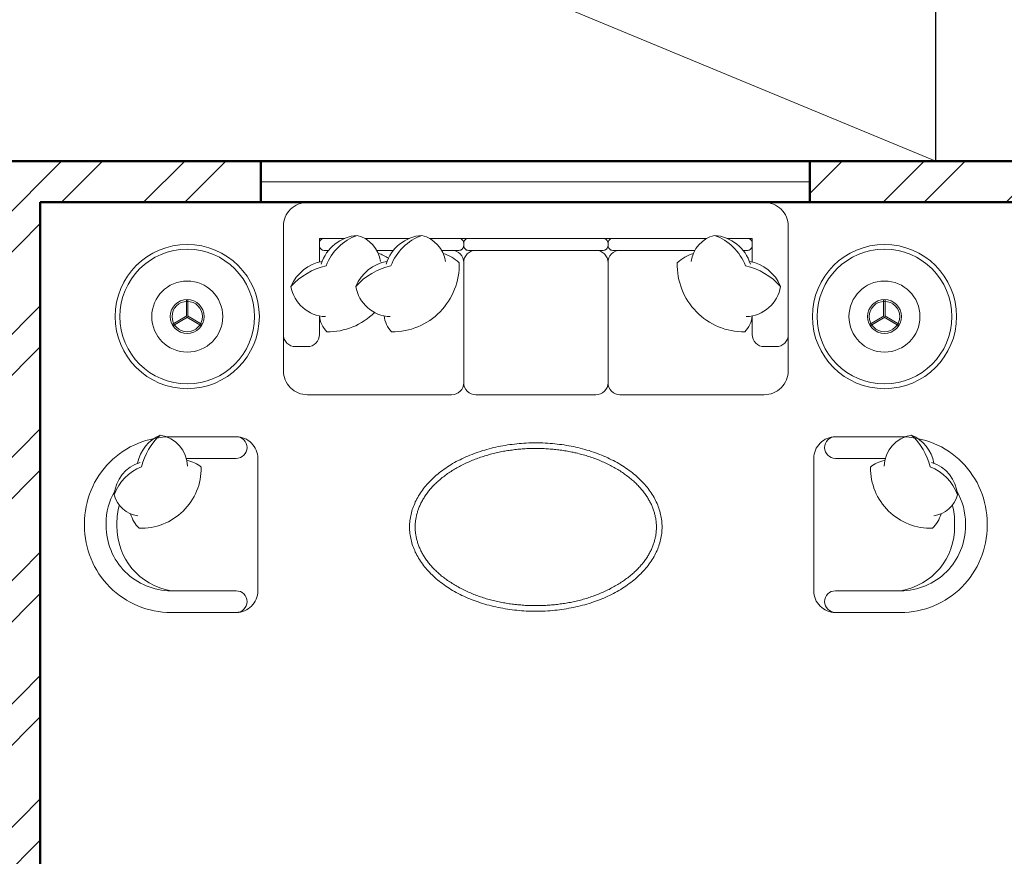
# Model space of a CAD drawing. Units: inches. Extents: x 1901 to 2863, y 888 to 2433.
# Tile 19 of 91: x 2157 to 2264, y 1641 to 1732. Entities that reach past the tile are written whole.
import ezdxf

# ---------------------------------------------------------------- set-up
doc = ezdxf.new("R2010")
doc.units = ezdxf.units.IN
for name, color, linetype, lineweight in [('A-ANNO-SYMB', 8, 'Continuous', 13), ('A-FLOR-HRAL', 41, 'Continuous', 25), ('A-FURN', 8, 'Continuous', 18), ('A-WALL', 7, 'Continuous', 50), ('A-WALL-PATT', 8, 'Continuous', 13)]:
    doc.layers.add(name, color=color, linetype=linetype, lineweight=lineweight)

msp = doc.modelspace()

# ---------------------------------------------------------------- hatches: boundary and pattern name
at = {"layer": 'A-WALL-PATT'}
h = msp.add_hatch(dxfattribs=at)
h.set_pattern_fill('ANSI32', color=256)
h.paths.add_polyline_path([(2182.93, 1716.63), (2024.93, 1716.63), (2024.93, 1681.7), (2029.33, 1681.7), (2029.33, 1712.13), (2154.33, 1712.13), (2154.33, 1580.13), (2148.52, 1580.13), (2148.52, 1577.88), (2148.52, 1575.63), (2194.93, 1575.63), (2194.93, 1580.13), (2158.83, 1580.13), (2158.83, 1712.13), (2182.93, 1712.13)])
h.paths.add_polyline_path([(2301.07, 1716.63), (2242.93, 1716.63), (2242.93, 1712.13), (2283.83, 1712.13), (2283.83, 1685.54), (2288.33, 1685.54), (2288.33, 1712.13), (2301.07, 1712.13)])
h.paths.add_polyline_path([(2288.33, 1600.41), (2286.08, 1600.41), (2283.83, 1600.41), (2283.83, 1580.13), (2270.6, 1580.13), (2270.6, 1575.63), (2288.33, 1575.63)])
h.paths.add_polyline_path([(2295.93, 1953.63), (2271.45, 1953.63), (2271.45, 1949.13), (2291.43, 1949.13), (2291.43, 1941.24), (2295.93, 1941.24)])
h.paths.add_polyline_path([(2098.38, 1244.13), (2082.33, 1244.13), (2082.33, 1302.13), (2086.52, 1302.13), (2086.52, 1306.63), (2067.46, 1306.63), (2067.46, 1302.13), (2077.83, 1302.13), (2077.83, 1239.63), (2098.38, 1239.63), (2098.38, 1241.88)])
h.paths.add_polyline_path([(2217.31, 1306.63), (2158.83, 1306.63), (2158.83, 1451.63), (2162.72, 1451.63), (2162.72, 1453.88), (2162.72, 1456.13), (2154.33, 1456.13), (2154.33, 1443.13), (2151.91, 1443.13), (2151.91, 1438.63), (2154.33, 1438.63), (2154.33, 1306.63), (2109.31, 1306.63), (2109.31, 1304.38), (2109.31, 1302.13), (2154.33, 1302.13), (2154.33, 1244.13), (2122.38, 1244.13), (2122.38, 1239.63), (2154.33, 1239.63), (2154.33, 1223.63), (2163.33, 1223.63), (2181.01, 1223.63), (2181.01, 1225.88), (2181.01, 1228.13), (2163.33, 1228.13), (2163.33, 1258.22), (2158.83, 1258.22), (2158.83, 1302.13), (2217.31, 1302.13)])
h.paths.add_polyline_path([(2259.99, 1306.63), (2238.3, 1306.63), (2238.3, 1304.38), (2238.3, 1302.13), (2242.83, 1302.13), (2242.83, 1228.13), (2205.01, 1228.13), (2205.01, 1223.63), (2247.33, 1223.63), (2247.33, 1302.13), (2259.99, 1302.13), (2259.99, 1304.38)])
h.paths.add_polyline_path([(2343.43, 1361.7), (2338.93, 1361.7), (2338.93, 1306.63), (2322.38, 1306.63), (2322.38, 1302.13), (2343.43, 1302.13)])
h.paths.add_polyline_path([(2343.43, 1470.4), (2338.93, 1470.4), (2338.93, 1456.13), (2193.73, 1456.13), (2193.73, 1453.88), (2193.73, 1451.63), (2338.93, 1451.63), (2338.93, 1421.7), (2343.43, 1421.7)])
h.paths.add_polyline_path([(2343.43, 1545.51), (2338.93, 1545.51), (2338.93, 1530.4), (2343.43, 1530.4)])
h.paths.add_polyline_path([(2029.33, 1466.83), (2024.93, 1466.83), (2024.93, 1409.82), (2029.33, 1409.82)])
h.paths.add_polyline_path([(2122.84, 1440.88), (2122.84, 1443.13), (2121.83, 1443.13), (2121.83, 1498.18), (2119.58, 1498.18), (2117.33, 1498.18), (2117.33, 1443.13), (2029.33, 1443.13), (2029.33, 1438.63), (2122.84, 1438.63)])
h.paths.add_polyline_path([(2029.33, 1543.05), (2024.93, 1543.05), (2024.93, 1502.83), (2029.33, 1502.83)])
h.paths.add_polyline_path([(2029.33, 1621.7), (2024.93, 1621.7), (2024.93, 1567.05), (2027.13, 1567.05), (2029.33, 1567.05), (2029.33, 1575.63), (2109.33, 1575.63), (2109.33, 1554.71), (2113.83, 1554.71), (2113.83, 1575.63), (2115.8, 1575.63), (2115.8, 1577.88), (2115.8, 1580.13), (2029.33, 1580.13)])
h.paths.add_polyline_path([(2121.83, 1527.63), (2117.33, 1527.63), (2113.83, 1527.63), (2113.83, 1533.01), (2111.58, 1533.01), (2109.33, 1533.01), (2109.33, 1527.63), (2029.33, 1527.63), (2029.33, 1523.13), (2117.33, 1523.13), (2117.33, 1519.43), (2121.83, 1519.43)])
h.paths.add_polyline_path([(2029.33, 1349.82), (2024.93, 1349.82), (2024.93, 1302.13), (2036.28, 1302.13), (2036.28, 1306.63), (2029.33, 1306.63)])

# ---------------------------------------------------------------- linework, layer by layer
at = {"layer": 'A-ANNO-SYMB'}
msp.add_line((2024.93, 1812.63), (2256.71, 1716.63), dxfattribs=at)
at = {"layer": 'A-FLOR-HRAL'}
msp.add_line((2256.71, 1716.63), (2256.71, 1812.63), dxfattribs=at)
at = {"layer": 'A-FURN'}
msp.add_line((2182.93, 1714.38), (2242.93, 1714.38), dxfattribs=at)
at = {"layer": 'A-FURN', "ltscale": 0.03}
for p, q in [((2174.8, 1699.65), (2174.8, 1701.5)), ((2174.97, 1699.65), (2174.97, 1701.5)), ((2251.01, 1699.65), (2251.01, 1701.5)), ((2251.18, 1699.65), (2251.18, 1701.5)), ((2174.84, 1699.72), (2173.24, 1698.8)), ((2174.93, 1699.58), (2173.32, 1698.65)), ((2174.84, 1699.58), (2176.45, 1698.65)), ((2174.93, 1699.72), (2176.53, 1698.8)), ((2251.06, 1699.72), (2249.45, 1698.8)), ((2251.14, 1699.58), (2249.53, 1698.65)), ((2251.06, 1699.58), (2252.66, 1698.65)), ((2251.14, 1699.72), (2252.74, 1698.8))]:
    msp.add_line(p, q, dxfattribs=at)
msp.add_lwpolyline([(2240.59, 1693.74, -0.414214), (2237.96, 1691.11), (2222.19, 1691.11, -0.414214), (2220.88, 1692.42, -0.414214), (2219.56, 1691.11), (2206.42, 1691.11, -0.414214), (2205.11, 1692.42, -0.414214), (2203.79, 1691.11), (2188.03, 1691.11, -0.414214), (2185.4, 1693.74), (2185.4, 1709.51, -0.414214), (2188.03, 1712.13), (2237.96, 1712.13, -0.414214), (2240.59, 1709.51)], format="xyb", close=True, dxfattribs=at)
at = {"layer": 'A-FURN'}
for points in [[(2186.23, 1702.95, -0.14773), (2190.07, 1705.21, -0.213343), (2193.46, 1708.52, -0.178662)], [(2192.1, 1708.19), (2189.34, 1708.19), (2189.34, 1705.61, -0.414214)], [(2190.34, 1706.88), (2189.86, 1706.88, -0.414214), (2189.34, 1707.4), (2189.34, 1707.67, -0.414214), (2189.86, 1708.19)], [(2189.54, 1705.39, -0.306663), (2193.46, 1708.52, -0.30633), (2196.02, 1705.66, 0.872847)], [(2189.86, 1708.19), (2192.1, 1708.19, -0.414214)], [(2193.31, 1702.95, -0.14773), (2197.15, 1705.21, -0.213343), (2200.54, 1708.52, -0.178662)], [(2194.29, 1708.19), (2199.18, 1708.19, -0.414214)], [(2196.62, 1705.39, -0.306663), (2200.54, 1708.52, -0.30633), (2203.1, 1705.66, 0.872847)], [(2201.37, 1708.19), (2204.58, 1708.19, -0.414214), (2205.11, 1707.67), (2205.11, 1707.4, -0.414214), (2204.58, 1706.88), (2202.69, 1706.88, -0.414214)], [(2231.69, 1708.19), (2221.4, 1708.19, 0.414214), (2220.88, 1707.67), (2220.88, 1707.4, 0.414214), (2221.4, 1706.88), (2230.37, 1706.88, 0.414214)], [(2236.44, 1705.39, 0.306663), (2232.52, 1708.52, 0.30633), (2229.96, 1705.66, -0.872847)], [(2239.75, 1702.95, 0.14773), (2235.91, 1705.21, 0.213343), (2232.52, 1708.52, 0.178662)], [(2236.12, 1708.19), (2233.88, 1708.19, 0.414214)], [(2235.64, 1706.88), (2236.12, 1706.88, 0.414214), (2236.64, 1707.4), (2236.64, 1707.67, 0.414214), (2236.12, 1708.19)], [(2197.42, 1706.88), (2195.61, 1706.88, -0.414214)], [(2203.79, 1706.88, -0.414214), (2205.11, 1705.56), (2205.11, 1692.42, -0.414214)], [(2206.42, 1706.88, 0.414214), (2205.11, 1705.56)], [(2219.56, 1706.88, -0.414214), (2220.88, 1705.56)], [(2222.19, 1706.88, 0.414214), (2220.88, 1705.56), (2220.88, 1692.42, 0.414214)], [(2196.88, 1706.03, 0.071865), (2195.78, 1706.55, -7.115464)], [(2196.41, 1699.72, 0.165541), (2197.23, 1697.98, 0.425989), (2204.61, 1705.51, 0.121523), (2202.86, 1706.55, -7.115464)], [(2236.65, 1699.72, -0.165541), (2235.83, 1697.98, -0.425989), (2228.45, 1705.51, -0.121523), (2230.21, 1706.55, 7.115464)], [(2190, 1699.64, -0.356772), (2186.23, 1702.95, -0.249542), (2189.65, 1705.68, 9.61688)], [(2197.08, 1699.64, -0.356772), (2193.31, 1702.95, -0.249542), (2196.72, 1705.68, 9.61688)], [(2235.98, 1699.64, 0.356772), (2239.75, 1702.95, 0.249542), (2236.34, 1705.68, -9.61688)], [(2189.34, 1699.72), (2189.34, 1697.68, -0.414214), (2188.03, 1696.37), (2186.71, 1696.37, -0.414214), (2185.4, 1697.68)], [(2189.34, 1699.72, 0.165541), (2190.15, 1697.98, 0.200231), (2195.37, 1700.09, 0.121523)], [(2240.59, 1697.68, -0.414214), (2239.27, 1696.37), (2237.96, 1696.37, -0.414214), (2236.64, 1697.68), (2236.64, 1699.72)], [(2171.94, 1686.71, 0.14773), (2169.9, 1683.25, 0.213343), (2166.91, 1680.19, 0.178662)], [(2174.92, 1683.31, 0.356772), (2171.94, 1686.71, 0.249542), (2169.47, 1683.63, -9.61688)], [(2174.79, 1684.15), (2180.24, 1684.15, 0.414214), (2181.43, 1685.33), (2181.43, 1685.33, 0.414214), (2180.24, 1686.52)], [(2251.19, 1684.15), (2245.74, 1684.15, -0.414214), (2244.56, 1685.33), (2244.56, 1685.33, -0.414214), (2245.74, 1686.52)], [(2251.06, 1683.31, -0.356772), (2254.05, 1686.71, -0.249542), (2256.51, 1683.63, 9.61688)], [(2254.05, 1686.71, -0.14773), (2256.08, 1683.25, -0.213343), (2259.07, 1680.19, -0.178662)], [(2169.74, 1683.72, 0.306663), (2166.91, 1680.19, 0.30633), (2169.49, 1677.88, -0.872847)], [(2174.85, 1683.91, -0.165541), (2176.42, 1683.18, -0.425989), (2169.63, 1676.52, -0.121523), (2168.69, 1678.1, 7.115464)], [(2251.13, 1683.91, 0.165541), (2249.57, 1683.18, 0.425989), (2256.35, 1676.52, 0.121523), (2257.29, 1678.1, -7.115464)], [(2256.24, 1683.72, -0.306663), (2259.07, 1680.19, -0.30633), (2256.49, 1677.88, 0.872847)], [(2166.96, 1680.57, 0.130591), (2166.02, 1677.04), (2166.02, 1676.92)], [(2259.02, 1680.57, -0.130591), (2259.96, 1677.04), (2259.96, 1676.92)], [(2167.46, 1679.06, 0.072384), (2167.21, 1677.04), (2167.21, 1676.92)], [(2258.52, 1679.06, -0.072384), (2258.77, 1677.04), (2258.77, 1676.92)], [(2173.13, 1669.69, -0.414214), (2166.02, 1676.8), (2166.02, 1676.92)], [(2173.13, 1669.69, -0.372719), (2167.21, 1676.8), (2167.21, 1676.92)], [(2252.85, 1669.69, 0.372719), (2258.77, 1676.8), (2258.77, 1676.92)], [(2252.85, 1669.69, 0.414214), (2259.96, 1676.8), (2259.96, 1676.92)], [(2173.13, 1669.69), (2180.24, 1669.69, -0.414214), (2181.43, 1668.51), (2181.43, 1668.51, -0.414214), (2180.24, 1667.32)], [(2252.85, 1669.69), (2245.74, 1669.69, 0.414214), (2244.56, 1668.51), (2244.56, 1668.51, 0.414214), (2245.74, 1667.32)]]:
    msp.add_lwpolyline(points, format="xyb", dxfattribs=at)
for points in [[(2199.18, 1708.19), (2194.29, 1708.19)], [(2231.69, 1708.19), (2201.37, 1708.19)], [(2236.64, 1705.61), (2236.64, 1708.19), (2233.88, 1708.19)]]:
    msp.add_lwpolyline(points, dxfattribs=at)
msp.add_lwpolyline([(2205.63, 1708.19), (2220.35, 1708.19, -0.414214), (2220.88, 1707.67), (2220.88, 1707.4, -0.414214), (2220.35, 1706.88), (2205.63, 1706.88, -0.414214), (2205.11, 1707.4), (2205.11, 1707.67, -0.414214)], format="xyb", close=True, dxfattribs=at)
at = {"layer": 'A-FURN', "ltscale": 0.03}
for points in [[(2182.61, 1676.92), (2182.61, 1669.69, -0.414214), (2180.24, 1667.32), (2173.13, 1667.32, -0.414214), (2163.65, 1676.8), (2163.65, 1676.92), (2163.65, 1677.04, -0.414214), (2173.13, 1686.52), (2180.24, 1686.52, -0.414214), (2182.61, 1684.15), (2182.61, 1676.92)], [(2243.37, 1676.92), (2243.37, 1669.69, 0.414214), (2245.74, 1667.32), (2252.85, 1667.32, 0.414214), (2262.33, 1676.8), (2262.33, 1676.92), (2262.33, 1677.04, 0.414214), (2252.85, 1686.52), (2245.74, 1686.52, 0.414214), (2243.37, 1684.15), (2243.37, 1676.92)]]:
    msp.add_lwpolyline(points, format="xyb", dxfattribs=at)
msp.add_polyline3d([(2226.79, 1676.66, 0), (2226.79, 1676.83, 0), (2226.78, 1677, 0), (2226.77, 1677.18, 0), (2226.75, 1677.35, 0), (2226.73, 1677.52, 0), (2226.7, 1677.7, 0), (2226.67, 1677.87, 0), (2226.63, 1678.04, 0), (2226.59, 1678.21, 0), (2226.54, 1678.39, 0), (2226.49, 1678.56, 0), (2226.43, 1678.73, 0), (2226.37, 1678.9, 0), (2226.31, 1679.06, 0), (2226.24, 1679.23, 0), (2226.16, 1679.4, 0), (2226.08, 1679.56, 0), (2226, 1679.73, 0), (2225.91, 1679.89, 0), (2225.81, 1680.05, 0), (2225.71, 1680.22, 0), (2225.61, 1680.38, 0), (2225.5, 1680.53, 0), (2225.39, 1680.69, 0), (2225.27, 1680.85, 0), (2225.15, 1681, 0), (2225.03, 1681.15, 0), (2224.9, 1681.3, 0), (2224.76, 1681.45, 0), (2224.62, 1681.6, 0), (2224.48, 1681.75, 0), (2224.33, 1681.89, 0), (2224.18, 1682.03, 0), (2224.03, 1682.17, 0), (2223.87, 1682.31, 0), (2223.71, 1682.45, 0), (2223.54, 1682.58, 0), (2223.37, 1682.71, 0), (2223.2, 1682.84, 0), (2223.02, 1682.97, 0), (2222.84, 1683.1, 0), (2222.65, 1683.22, 0), (2222.47, 1683.34, 0), (2222.27, 1683.46, 0), (2222.08, 1683.58, 0), (2221.88, 1683.69, 0), (2221.68, 1683.8, 0), (2221.48, 1683.91, 0), (2221.27, 1684.01, 0), (2221.06, 1684.12, 0), (2220.85, 1684.22, 0), (2220.63, 1684.32, 0), (2220.41, 1684.41, 0), (2220.19, 1684.5, 0), (2219.96, 1684.59, 0), (2219.74, 1684.68, 0), (2219.51, 1684.76, 0), (2219.28, 1684.84, 0), (2219.04, 1684.92, 0), (2218.81, 1685, 0), (2218.57, 1685.07, 0), (2218.33, 1685.14, 0), (2218.09, 1685.2, 0), (2217.85, 1685.27, 0), (2217.6, 1685.33, 0), (2217.35, 1685.38, 0), (2217.11, 1685.44, 0), (2216.86, 1685.49, 0), (2216.6, 1685.53, 0), (2216.35, 1685.58, 0), (2216.1, 1685.62, 0), (2215.84, 1685.66, 0), (2215.59, 1685.69, 0), (2215.33, 1685.72, 0), (2215.07, 1685.75, 0), (2214.81, 1685.77, 0), (2214.55, 1685.79, 0), (2214.29, 1685.81, 0), (2214.03, 1685.83, 0), (2213.77, 1685.84, 0), (2213.51, 1685.85, 0), (2213.25, 1685.85, 0), (2212.99, 1685.85, 0), (2212.73, 1685.85, 0), (2212.47, 1685.85, 0), (2212.21, 1685.84, 0), (2211.95, 1685.83, 0), (2211.69, 1685.81, 0), (2211.43, 1685.79, 0), (2211.17, 1685.77, 0), (2210.91, 1685.75, 0), (2210.65, 1685.72, 0), (2210.4, 1685.69, 0), (2210.14, 1685.66, 0), (2209.88, 1685.62, 0), (2209.63, 1685.58, 0), (2209.38, 1685.53, 0), (2209.13, 1685.49, 0), (2208.88, 1685.44, 0), (2208.63, 1685.38, 0), (2208.38, 1685.33, 0), (2208.14, 1685.27, 0), (2207.89, 1685.2, 0), (2207.65, 1685.14, 0), (2207.41, 1685.07, 0), (2207.17, 1685, 0), (2206.94, 1684.92, 0), (2206.7, 1684.84, 0), (2206.47, 1684.76, 0), (2206.24, 1684.68, 0), (2206.02, 1684.59, 0), (2205.79, 1684.5, 0), (2205.57, 1684.41, 0), (2205.35, 1684.32, 0), (2205.14, 1684.22, 0), (2204.92, 1684.12, 0), (2204.71, 1684.01, 0), (2204.51, 1683.91, 0), (2204.3, 1683.8, 0), (2204.1, 1683.69, 0), (2203.9, 1683.58, 0), (2203.71, 1683.46, 0), (2203.52, 1683.34, 0), (2203.33, 1683.22, 0), (2203.14, 1683.1, 0), (2202.96, 1682.97, 0), (2202.78, 1682.84, 0), (2202.61, 1682.71, 0), (2202.44, 1682.58, 0), (2202.27, 1682.45, 0), (2202.11, 1682.31, 0), (2201.95, 1682.17, 0), (2201.8, 1682.03, 0), (2201.65, 1681.89, 0), (2201.5, 1681.75, 0), (2201.36, 1681.6, 0), (2201.22, 1681.45, 0), (2201.09, 1681.3, 0), (2200.96, 1681.15, 0), (2200.83, 1681, 0), (2200.71, 1680.85, 0), (2200.59, 1680.69, 0), (2200.48, 1680.53, 0), (2200.37, 1680.38, 0), (2200.27, 1680.22, 0), (2200.17, 1680.05, 0), (2200.08, 1679.89, 0), (2199.99, 1679.73, 0), (2199.9, 1679.56, 0), (2199.82, 1679.4, 0), (2199.75, 1679.23, 0), (2199.68, 1679.06, 0), (2199.61, 1678.9, 0), (2199.55, 1678.73, 0), (2199.49, 1678.56, 0), (2199.44, 1678.39, 0), (2199.39, 1678.21, 0), (2199.35, 1678.04, 0), (2199.32, 1677.87, 0), (2199.28, 1677.7, 0), (2199.26, 1677.52, 0), (2199.23, 1677.35, 0), (2199.22, 1677.18, 0), (2199.2, 1677, 0), (2199.2, 1676.83, 0), (2199.19, 1676.66, 0), (2199.2, 1676.48, 0), (2199.2, 1676.31, 0), (2199.22, 1676.13, 0), (2199.23, 1675.96, 0), (2199.26, 1675.79, 0), (2199.28, 1675.61, 0), (2199.32, 1675.44, 0), (2199.35, 1675.27, 0), (2199.39, 1675.1, 0), (2199.44, 1674.93, 0), (2199.49, 1674.75, 0), (2199.55, 1674.58, 0), (2199.61, 1674.42, 0), (2199.68, 1674.25, 0), (2199.75, 1674.08, 0), (2199.82, 1673.91, 0), (2199.9, 1673.75, 0), (2199.99, 1673.58, 0), (2200.08, 1673.42, 0), (2200.17, 1673.26, 0), (2200.27, 1673.1, 0), (2200.37, 1672.94, 0), (2200.48, 1672.78, 0), (2200.59, 1672.62, 0), (2200.71, 1672.46, 0), (2200.83, 1672.31, 0), (2200.96, 1672.16, 0), (2201.09, 1672.01, 0), (2201.22, 1671.86, 0), (2201.36, 1671.71, 0), (2201.5, 1671.56, 0), (2201.65, 1671.42, 0), (2201.8, 1671.28, 0), (2201.95, 1671.14, 0), (2202.11, 1671, 0), (2202.27, 1670.86, 0), (2202.44, 1670.73, 0), (2202.61, 1670.6, 0), (2202.78, 1670.47, 0), (2202.96, 1670.34, 0), (2203.14, 1670.21, 0), (2203.33, 1670.09, 0), (2203.52, 1669.97, 0), (2203.71, 1669.85, 0), (2203.9, 1669.74, 0), (2204.1, 1669.62, 0), (2204.3, 1669.51, 0), (2204.51, 1669.4, 0), (2204.71, 1669.3, 0), (2204.92, 1669.19, 0), (2205.14, 1669.09, 0), (2205.35, 1669, 0), (2205.57, 1668.9, 0), (2205.79, 1668.81, 0), (2206.02, 1668.72, 0), (2206.24, 1668.63, 0), (2206.47, 1668.55, 0), (2206.7, 1668.47, 0), (2206.94, 1668.39, 0), (2207.17, 1668.32, 0), (2207.41, 1668.24, 0), (2207.65, 1668.17, 0), (2207.89, 1668.11, 0), (2208.14, 1668.05, 0), (2208.38, 1667.99, 0), (2208.63, 1667.93, 0), (2208.88, 1667.88, 0), (2209.13, 1667.83, 0), (2209.38, 1667.78, 0), (2209.63, 1667.73, 0), (2209.88, 1667.69, 0), (2210.14, 1667.66, 0), (2210.4, 1667.62, 0), (2210.65, 1667.59, 0), (2210.91, 1667.56, 0), (2211.17, 1667.54, 0), (2211.43, 1667.52, 0), (2211.69, 1667.5, 0), (2211.95, 1667.48, 0), (2212.21, 1667.47, 0), (2212.47, 1667.46, 0), (2212.73, 1667.46, 0), (2212.99, 1667.46, 0), (2213.25, 1667.46, 0), (2213.51, 1667.46, 0), (2213.77, 1667.47, 0), (2214.03, 1667.48, 0), (2214.29, 1667.5, 0), (2214.55, 1667.52, 0), (2214.81, 1667.54, 0), (2215.07, 1667.56, 0), (2215.33, 1667.59, 0), (2215.59, 1667.62, 0), (2215.84, 1667.66, 0), (2216.1, 1667.69, 0), (2216.35, 1667.73, 0), (2216.6, 1667.78, 0), (2216.86, 1667.83, 0), (2217.11, 1667.88, 0), (2217.35, 1667.93, 0), (2217.6, 1667.99, 0), (2217.85, 1668.05, 0), (2218.09, 1668.11, 0), (2218.33, 1668.17, 0), (2218.57, 1668.24, 0), (2218.81, 1668.32, 0), (2219.04, 1668.39, 0), (2219.28, 1668.47, 0), (2219.51, 1668.55, 0), (2219.74, 1668.63, 0), (2219.96, 1668.72, 0), (2220.19, 1668.81, 0), (2220.41, 1668.9, 0), (2220.63, 1669, 0), (2220.85, 1669.09, 0), (2221.06, 1669.19, 0), (2221.27, 1669.3, 0), (2221.48, 1669.4, 0), (2221.68, 1669.51, 0), (2221.88, 1669.62, 0), (2222.08, 1669.74, 0), (2222.27, 1669.85, 0), (2222.47, 1669.97, 0), (2222.65, 1670.09, 0), (2222.84, 1670.21, 0), (2223.02, 1670.34, 0), (2223.2, 1670.47, 0), (2223.37, 1670.6, 0), (2223.54, 1670.73, 0), (2223.71, 1670.86, 0), (2223.87, 1671, 0), (2224.03, 1671.14, 0), (2224.18, 1671.28, 0), (2224.33, 1671.42, 0), (2224.48, 1671.56, 0), (2224.62, 1671.71, 0), (2224.76, 1671.86, 0), (2224.9, 1672.01, 0), (2225.03, 1672.16, 0), (2225.15, 1672.31, 0), (2225.27, 1672.46, 0), (2225.39, 1672.62, 0), (2225.5, 1672.78, 0), (2225.61, 1672.94, 0), (2225.71, 1673.1, 0), (2225.81, 1673.26, 0), (2225.91, 1673.42, 0), (2226, 1673.58, 0), (2226.08, 1673.75, 0), (2226.16, 1673.91, 0), (2226.24, 1674.08, 0), (2226.31, 1674.25, 0), (2226.37, 1674.42, 0), (2226.43, 1674.58, 0), (2226.49, 1674.75, 0), (2226.54, 1674.93, 0), (2226.59, 1675.1, 0), (2226.63, 1675.27, 0), (2226.67, 1675.44, 0), (2226.7, 1675.61, 0), (2226.73, 1675.79, 0), (2226.75, 1675.96, 0), (2226.77, 1676.13, 0), (2226.78, 1676.31, 0), (2226.79, 1676.48, 0), (2226.79, 1676.66, 0)], dxfattribs=at)
at = {"layer": 'A-FURN'}
msp.add_polyline3d([(2226.18, 1676.66, 0), (2226.17, 1676.75, 0), (2226.17, 1676.84, 0), (2226.17, 1676.94, 0), (2226.16, 1677.03, 0), (2226.15, 1677.13, 0), (2226.15, 1677.23, 0), (2226.13, 1677.32, 0), (2226.12, 1677.42, 0), (2226.11, 1677.52, 0), (2226.09, 1677.61, 0), (2226.07, 1677.71, 0), (2226.05, 1677.81, 0), (2226.03, 1677.91, 0), (2226.01, 1678.01, 0), (2225.98, 1678.11, 0), (2225.96, 1678.21, 0), (2225.93, 1678.31, 0), (2225.9, 1678.4, 0), (2225.86, 1678.5, 0), (2225.83, 1678.6, 0), (2225.79, 1678.7, 0), (2225.75, 1678.81, 0), (2225.71, 1678.91, 0), (2225.67, 1679.01, 0), (2225.62, 1679.11, 0), (2225.57, 1679.21, 0), (2225.52, 1679.31, 0), (2225.47, 1679.41, 0), (2225.42, 1679.51, 0), (2225.36, 1679.61, 0), (2225.3, 1679.71, 0), (2225.24, 1679.81, 0), (2225.18, 1679.91, 0), (2225.11, 1680.01, 0), (2225.05, 1680.11, 0), (2224.98, 1680.21, 0), (2224.91, 1680.31, 0), (2224.84, 1680.41, 0), (2224.76, 1680.51, 0), (2224.68, 1680.6, 0), (2224.6, 1680.7, 0), (2224.52, 1680.8, 0), (2224.44, 1680.9, 0), (2224.35, 1680.99, 0), (2224.26, 1681.09, 0), (2224.17, 1681.18, 0), (2224.08, 1681.28, 0), (2223.99, 1681.37, 0), (2223.89, 1681.47, 0), (2223.79, 1681.56, 0), (2223.69, 1681.65, 0), (2223.58, 1681.74, 0), (2223.48, 1681.83, 0), (2223.37, 1681.92, 0), (2223.26, 1682.01, 0), (2223.15, 1682.1, 0), (2223.04, 1682.19, 0), (2222.92, 1682.27, 0), (2222.81, 1682.36, 0), (2222.69, 1682.45, 0), (2222.57, 1682.53, 0), (2222.45, 1682.61, 0), (2222.32, 1682.69, 0), (2222.2, 1682.78, 0), (2222.07, 1682.86, 0), (2221.94, 1682.93, 0), (2221.81, 1683.01, 0), (2221.68, 1683.09, 0), (2221.55, 1683.17, 0), (2221.41, 1683.24, 0), (2221.28, 1683.31, 0), (2221.14, 1683.39, 0), (2221, 1683.46, 0), (2220.86, 1683.53, 0), (2220.72, 1683.6, 0), (2220.58, 1683.66, 0), (2220.44, 1683.73, 0), (2220.29, 1683.79, 0), (2220.14, 1683.86, 0), (2220, 1683.92, 0), (2219.85, 1683.98, 0), (2219.7, 1684.04, 0), (2219.55, 1684.09, 0), (2219.4, 1684.15, 0), (2219.25, 1684.21, 0), (2219.09, 1684.26, 0), (2218.94, 1684.31, 0), (2218.79, 1684.36, 0), (2218.64, 1684.41, 0), (2218.48, 1684.46, 0), (2218.33, 1684.5, 0), (2218.17, 1684.55, 0), (2218.02, 1684.59, 0), (2217.86, 1684.63, 0), (2217.71, 1684.67, 0), (2217.55, 1684.71, 0), (2217.4, 1684.75, 0), (2217.24, 1684.78, 0), (2217.08, 1684.82, 0), (2216.93, 1684.85, 0), (2216.77, 1684.88, 0), (2216.61, 1684.91, 0), (2216.46, 1684.94, 0), (2216.3, 1684.97, 0), (2216.14, 1684.99, 0), (2215.98, 1685.02, 0), (2215.82, 1685.04, 0), (2215.66, 1685.06, 0), (2215.51, 1685.08, 0), (2215.35, 1685.1, 0), (2215.19, 1685.12, 0), (2215.03, 1685.14, 0), (2214.87, 1685.15, 0), (2214.71, 1685.17, 0), (2214.55, 1685.18, 0), (2214.39, 1685.19, 0), (2214.23, 1685.2, 0), (2214.07, 1685.21, 0), (2213.91, 1685.22, 0), (2213.75, 1685.23, 0), (2213.59, 1685.23, 0), (2213.43, 1685.24, 0), (2213.27, 1685.24, 0), (2213.11, 1685.24, 0), (2212.95, 1685.24, 0), (2212.79, 1685.24, 0), (2212.63, 1685.24, 0), (2212.47, 1685.23, 0), (2212.31, 1685.23, 0), (2212.15, 1685.22, 0), (2211.99, 1685.22, 0), (2211.83, 1685.21, 0), (2211.67, 1685.2, 0), (2211.51, 1685.19, 0), (2211.35, 1685.18, 0), (2211.19, 1685.16, 0), (2211.03, 1685.15, 0), (2210.87, 1685.13, 0), (2210.71, 1685.11, 0), (2210.56, 1685.09, 0), (2210.4, 1685.07, 0), (2210.24, 1685.05, 0), (2210.08, 1685.03, 0), (2209.92, 1685.01, 0), (2209.76, 1684.98, 0), (2209.61, 1684.95, 0), (2209.45, 1684.93, 0), (2209.29, 1684.9, 0), (2209.13, 1684.86, 0), (2208.98, 1684.83, 0), (2208.82, 1684.8, 0), (2208.66, 1684.76, 0), (2208.51, 1684.73, 0), (2208.35, 1684.69, 0), (2208.2, 1684.65, 0), (2208.04, 1684.61, 0), (2207.89, 1684.57, 0), (2207.73, 1684.52, 0), (2207.58, 1684.48, 0), (2207.42, 1684.43, 0), (2207.27, 1684.38, 0), (2207.12, 1684.34, 0), (2206.96, 1684.28, 0), (2206.81, 1684.23, 0), (2206.66, 1684.18, 0), (2206.51, 1684.12, 0), (2206.36, 1684.07, 0), (2206.21, 1684.01, 0), (2206.06, 1683.95, 0), (2205.91, 1683.89, 0), (2205.76, 1683.82, 0), (2205.62, 1683.76, 0), (2205.48, 1683.7, 0), (2205.33, 1683.63, 0), (2205.19, 1683.56, 0), (2205.05, 1683.49, 0), (2204.91, 1683.42, 0), (2204.77, 1683.35, 0), (2204.64, 1683.28, 0), (2204.5, 1683.2, 0), (2204.37, 1683.13, 0), (2204.23, 1683.05, 0), (2204.1, 1682.97, 0), (2203.98, 1682.9, 0), (2203.85, 1682.82, 0), (2203.72, 1682.74, 0), (2203.6, 1682.65, 0), (2203.47, 1682.57, 0), (2203.35, 1682.49, 0), (2203.23, 1682.4, 0), (2203.12, 1682.32, 0), (2203, 1682.23, 0), (2202.89, 1682.14, 0), (2202.77, 1682.06, 0), (2202.66, 1681.97, 0), (2202.56, 1681.88, 0), (2202.45, 1681.79, 0), (2202.35, 1681.7, 0), (2202.24, 1681.6, 0), (2202.14, 1681.51, 0), (2202.05, 1681.42, 0), (2201.95, 1681.33, 0), (2201.86, 1681.23, 0), (2201.76, 1681.14, 0), (2201.67, 1681.04, 0), (2201.59, 1680.94, 0), (2201.5, 1680.85, 0), (2201.42, 1680.75, 0), (2201.34, 1680.65, 0), (2201.26, 1680.56, 0), (2201.18, 1680.46, 0), (2201.11, 1680.36, 0), (2201.04, 1680.26, 0), (2200.97, 1680.16, 0), (2200.9, 1680.06, 0), (2200.84, 1679.96, 0), (2200.77, 1679.86, 0), (2200.71, 1679.76, 0), (2200.65, 1679.66, 0), (2200.59, 1679.56, 0), (2200.54, 1679.46, 0), (2200.49, 1679.36, 0), (2200.44, 1679.26, 0), (2200.39, 1679.16, 0), (2200.34, 1679.06, 0), (2200.3, 1678.96, 0), (2200.25, 1678.86, 0), (2200.21, 1678.76, 0), (2200.17, 1678.65, 0), (2200.14, 1678.55, 0), (2200.1, 1678.45, 0), (2200.07, 1678.35, 0), (2200.04, 1678.26, 0), (2200.01, 1678.16, 0), (2199.99, 1678.06, 0), (2199.96, 1677.96, 0), (2199.94, 1677.86, 0), (2199.92, 1677.76, 0), (2199.9, 1677.66, 0), (2199.88, 1677.57, 0), (2199.87, 1677.47, 0), (2199.85, 1677.37, 0), (2199.84, 1677.27, 0), (2199.83, 1677.18, 0), (2199.82, 1677.08, 0), (2199.82, 1676.99, 0), (2199.81, 1676.89, 0), (2199.81, 1676.8, 0), (2199.81, 1676.7, 0), (2199.81, 1676.61, 0), (2199.81, 1676.51, 0), (2199.81, 1676.42, 0), (2199.82, 1676.32, 0), (2199.82, 1676.23, 0), (2199.83, 1676.13, 0), (2199.84, 1676.04, 0), (2199.85, 1675.94, 0), (2199.87, 1675.84, 0), (2199.88, 1675.75, 0), (2199.9, 1675.65, 0), (2199.92, 1675.55, 0), (2199.94, 1675.45, 0), (2199.96, 1675.35, 0), (2199.99, 1675.25, 0), (2200.01, 1675.16, 0), (2200.04, 1675.06, 0), (2200.07, 1674.96, 0), (2200.1, 1674.86, 0), (2200.14, 1674.76, 0), (2200.17, 1674.66, 0), (2200.21, 1674.56, 0), (2200.25, 1674.46, 0), (2200.3, 1674.36, 0), (2200.34, 1674.25, 0), (2200.39, 1674.15, 0), (2200.44, 1674.05, 0), (2200.49, 1673.95, 0), (2200.54, 1673.85, 0), (2200.59, 1673.75, 0), (2200.65, 1673.65, 0), (2200.71, 1673.55, 0), (2200.77, 1673.45, 0), (2200.84, 1673.35, 0), (2200.9, 1673.25, 0), (2200.97, 1673.15, 0), (2201.04, 1673.05, 0), (2201.11, 1672.95, 0), (2201.18, 1672.85, 0), (2201.26, 1672.76, 0), (2201.34, 1672.66, 0), (2201.42, 1672.56, 0), (2201.5, 1672.46, 0), (2201.59, 1672.37, 0), (2201.67, 1672.27, 0), (2201.76, 1672.18, 0), (2201.86, 1672.08, 0), (2201.95, 1671.99, 0), (2202.05, 1671.89, 0), (2202.14, 1671.8, 0), (2202.24, 1671.71, 0), (2202.35, 1671.62, 0), (2202.45, 1671.52, 0), (2202.56, 1671.43, 0), (2202.66, 1671.34, 0), (2202.77, 1671.26, 0), (2202.89, 1671.17, 0), (2203, 1671.08, 0), (2203.12, 1670.99, 0), (2203.23, 1670.91, 0), (2203.35, 1670.82, 0), (2203.47, 1670.74, 0), (2203.6, 1670.66, 0), (2203.72, 1670.58, 0), (2203.85, 1670.5, 0), (2203.98, 1670.42, 0), (2204.1, 1670.34, 0), (2204.23, 1670.26, 0), (2204.37, 1670.18, 0), (2204.5, 1670.11, 0), (2204.64, 1670.03, 0), (2204.77, 1669.96, 0), (2204.91, 1669.89, 0), (2205.05, 1669.82, 0), (2205.19, 1669.75, 0), (2205.33, 1669.68, 0), (2205.48, 1669.62, 0), (2205.62, 1669.55, 0), (2205.76, 1669.49, 0), (2205.91, 1669.42, 0), (2206.06, 1669.36, 0), (2206.21, 1669.3, 0), (2206.36, 1669.25, 0), (2206.51, 1669.19, 0), (2206.66, 1669.13, 0), (2206.81, 1669.08, 0), (2206.96, 1669.03, 0), (2207.12, 1668.98, 0), (2207.27, 1668.93, 0), (2207.42, 1668.88, 0), (2207.58, 1668.83, 0), (2207.73, 1668.79, 0), (2207.89, 1668.74, 0), (2208.04, 1668.7, 0), (2208.2, 1668.66, 0), (2208.35, 1668.62, 0), (2208.51, 1668.58, 0), (2208.66, 1668.55, 0), (2208.82, 1668.51, 0), (2208.98, 1668.48, 0), (2209.13, 1668.45, 0), (2209.29, 1668.42, 0), (2209.45, 1668.39, 0), (2209.61, 1668.36, 0), (2209.76, 1668.33, 0), (2209.92, 1668.31, 0), (2210.08, 1668.28, 0), (2210.24, 1668.26, 0), (2210.4, 1668.24, 0), (2210.56, 1668.22, 0), (2210.71, 1668.2, 0), (2210.87, 1668.18, 0), (2211.03, 1668.16, 0), (2211.19, 1668.15, 0), (2211.35, 1668.14, 0), (2211.51, 1668.12, 0), (2211.67, 1668.11, 0), (2211.83, 1668.1, 0), (2211.99, 1668.1, 0), (2212.15, 1668.09, 0), (2212.31, 1668.08, 0), (2212.47, 1668.08, 0), (2212.63, 1668.07, 0), (2212.79, 1668.07, 0), (2212.95, 1668.07, 0), (2213.11, 1668.07, 0), (2213.27, 1668.07, 0), (2213.43, 1668.08, 0), (2213.59, 1668.08, 0), (2213.75, 1668.08, 0), (2213.91, 1668.09, 0), (2214.07, 1668.1, 0), (2214.23, 1668.11, 0), (2214.39, 1668.12, 0), (2214.55, 1668.13, 0), (2214.71, 1668.14, 0), (2214.87, 1668.16, 0), (2215.03, 1668.17, 0), (2215.19, 1668.19, 0), (2215.35, 1668.21, 0), (2215.51, 1668.23, 0), (2215.66, 1668.25, 0), (2215.82, 1668.27, 0), (2215.98, 1668.29, 0), (2216.14, 1668.32, 0), (2216.3, 1668.34, 0), (2216.46, 1668.37, 0), (2216.61, 1668.4, 0), (2216.77, 1668.43, 0), (2216.93, 1668.46, 0), (2217.08, 1668.5, 0), (2217.24, 1668.53, 0), (2217.4, 1668.57, 0), (2217.55, 1668.6, 0), (2217.71, 1668.64, 0), (2217.86, 1668.68, 0), (2218.02, 1668.72, 0), (2218.17, 1668.77, 0), (2218.33, 1668.81, 0), (2218.48, 1668.86, 0), (2218.64, 1668.9, 0), (2218.79, 1668.95, 0), (2218.94, 1669, 0), (2219.09, 1669.05, 0), (2219.25, 1669.11, 0), (2219.4, 1669.16, 0), (2219.55, 1669.22, 0), (2219.7, 1669.27, 0), (2219.85, 1669.33, 0), (2220, 1669.39, 0), (2220.14, 1669.46, 0), (2220.29, 1669.52, 0), (2220.44, 1669.58, 0), (2220.58, 1669.65, 0), (2220.72, 1669.72, 0), (2220.86, 1669.78, 0), (2221, 1669.85, 0), (2221.14, 1669.93, 0), (2221.28, 1670, 0), (2221.41, 1670.07, 0), (2221.55, 1670.15, 0), (2221.68, 1670.22, 0), (2221.81, 1670.3, 0), (2221.94, 1670.38, 0), (2222.07, 1670.46, 0), (2222.2, 1670.54, 0), (2222.32, 1670.62, 0), (2222.45, 1670.7, 0), (2222.57, 1670.78, 0), (2222.69, 1670.87, 0), (2222.81, 1670.95, 0), (2222.92, 1671.04, 0), (2223.04, 1671.12, 0), (2223.15, 1671.21, 0), (2223.26, 1671.3, 0), (2223.37, 1671.39, 0), (2223.48, 1671.48, 0), (2223.58, 1671.57, 0), (2223.69, 1671.66, 0), (2223.79, 1671.75, 0), (2223.89, 1671.85, 0), (2223.99, 1671.94, 0), (2224.08, 1672.03, 0), (2224.17, 1672.13, 0), (2224.26, 1672.22, 0), (2224.35, 1672.32, 0), (2224.44, 1672.42, 0), (2224.52, 1672.51, 0), (2224.6, 1672.61, 0), (2224.68, 1672.71, 0), (2224.76, 1672.8, 0), (2224.84, 1672.9, 0), (2224.91, 1673, 0), (2224.98, 1673.1, 0), (2225.05, 1673.2, 0), (2225.11, 1673.3, 0), (2225.18, 1673.4, 0), (2225.24, 1673.5, 0), (2225.3, 1673.6, 0), (2225.36, 1673.7, 0), (2225.42, 1673.8, 0), (2225.47, 1673.9, 0), (2225.52, 1674, 0), (2225.57, 1674.1, 0), (2225.62, 1674.2, 0), (2225.67, 1674.31, 0), (2225.71, 1674.41, 0), (2225.75, 1674.51, 0), (2225.79, 1674.61, 0), (2225.83, 1674.71, 0), (2225.86, 1674.81, 0), (2225.9, 1674.91, 0), (2225.93, 1675.01, 0), (2225.96, 1675.11, 0), (2225.98, 1675.21, 0), (2226.01, 1675.3, 0), (2226.03, 1675.4, 0), (2226.05, 1675.5, 0), (2226.07, 1675.6, 0), (2226.09, 1675.7, 0), (2226.11, 1675.79, 0), (2226.12, 1675.89, 0), (2226.13, 1675.99, 0), (2226.15, 1676.09, 0), (2226.15, 1676.18, 0), (2226.16, 1676.28, 0), (2226.17, 1676.37, 0), (2226.17, 1676.47, 0), (2226.17, 1676.56, 0), (2226.18, 1676.66, 0)], dxfattribs=at)
at = {"layer": 'A-FURN', "ltscale": 0.03}
for centre, radius in [((2174.89, 1699.65), 7.88), ((2251.1, 1699.65), 7.88), ((2174.89, 1699.65), 3.88), ((2251.1, 1699.65), 3.88), ((2174.89, 1699.65), 1.85), ((2251.1, 1699.65), 1.85), ((2174.89, 1699.65), 1.66), ((2251.1, 1699.65), 1.66)]:
    msp.add_circle(centre, radius, dxfattribs=at)
at = {"layer": 'A-FURN'}
for centre in [(2174.89, 1699.65), (2251.1, 1699.65)]:
    msp.add_circle(centre, 7.36, dxfattribs=at)
at = {"layer": 'A-WALL'}
for p, q in [((2024.93, 1716.63), (2301.07, 1716.63)), ((2182.93, 1712.13), (2182.93, 1716.63)), ((2182.93, 1716.63), (2182.93, 1714.38)), ((2242.93, 1714.38), (2242.93, 1716.63)), ((2242.93, 1716.63), (2242.93, 1712.13)), ((2158.83, 1712.13), (2158.83, 1580.13)), ((2283.83, 1712.13), (2158.83, 1712.13))]:
    msp.add_line(p, q, dxfattribs=at)

doc.saveas('drawing.dxf')
